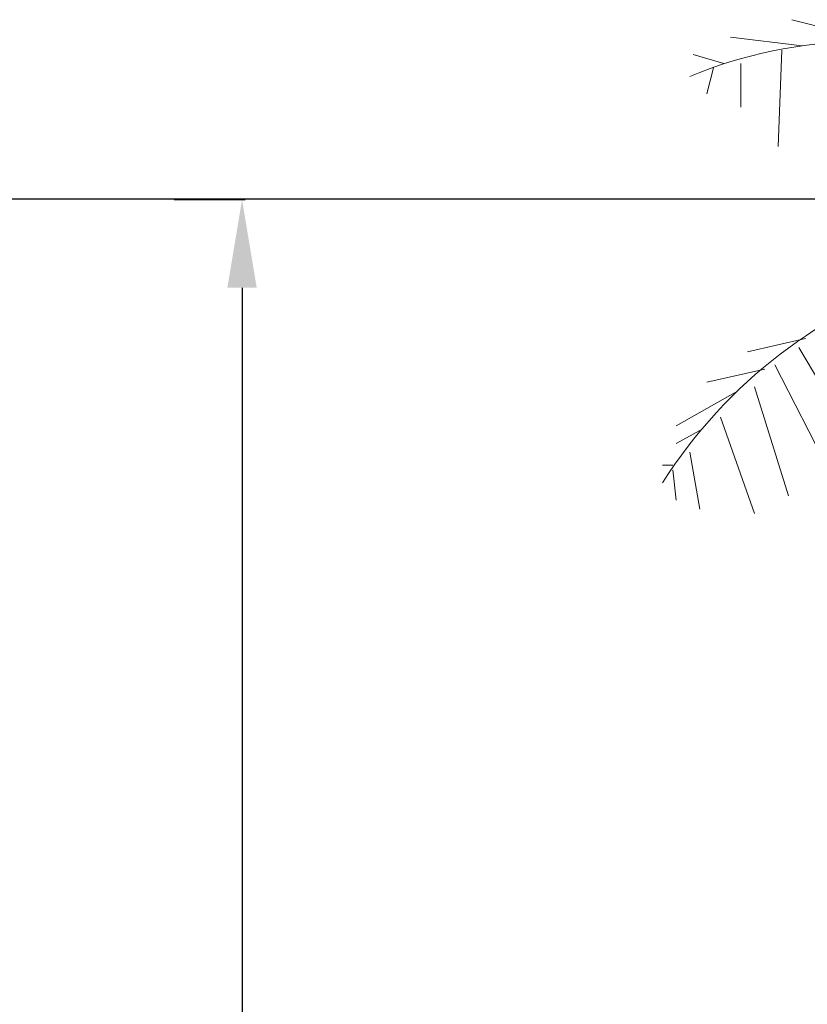
# Model space of a CAD drawing. Units: inches. Extents: x -301 to 715, y -607 to 364.
# Tile 51 of 141: x 150 to 194, y -370 to -314. Entities that reach past the tile are written whole.
import ezdxf

# ---------------------------------------------------------------- set-up
doc = ezdxf.new("R2010")
doc.units = ezdxf.units.IN
doc.header["$MEASUREMENT"] = 0
doc.layers.add('A-ANNO-DIMS', color=2, linetype='Continuous', lineweight=18)
doc.layers.add('L-PLNT', color=94, linetype='Continuous', lineweight=13)
doc.styles.get("Standard").update_dxf_attribs({"font": 'arial.ttf'})
doc.dimstyles.get("Standard").update_dxf_attribs({"dimtxt": 0.18, "dimasz": 0.18, "dimexe": 0.18, "dimexo": 0.0625, "dimgap": 0.09, "dimtad": 0, "dimtih": 1, "dimtoh": 1, "dimdec": 1, "dimzin": 0, "dimdsep": 46, "dimlunit": 4, "dimtxsty": 'Standard', "dimcen": 0.09, "dimclrd": 3, "dimclre": 4, "dimclrt": 6, "dimadec": 0, "dimazin": 0, "dimtfac": 1, "dimtdec": 1, "dimtofl": 0, "dimtmove": 0, "dimatfit": 3, "dimfxl": 1, "dimtfill": 2, "dimtfillclr": 51, "dimtolj": 1, "dimtzin": 0, "dimarcsym": 0})

# ---------------------------------------------------------------- blocks, each defined once
blk = doc.blocks.new('*U34')
for p, q in [((-20.064, 191.751), (-25.863, 193.238)), ((-25.283, 191.751), (-29.342, 192.246)), ((-29.729, 190.759), (-31.469, 191.255)), ((-26.443, 191.503), (-26.636, 186.051)), ((-30.309, 190.512), (-30.695, 189.025)), ((-28.763, 190.759), (-28.763, 188.281)), ((-25.09, 175.148), (-28.376, 174.404)), ((-25.476, 174.652), (-21.224, 167.466)), ((-27.409, 173.413), (-30.695, 172.67)), ((-26.829, 173.661), (-23.544, 167.218)), ((-28.956, 172.174), (-32.435, 170.192)), ((-27.989, 172.422), (-26.056, 166.227)), ((-29.922, 170.687), (-27.989, 165.235)), ((-31.082, 169.944), (-32.435, 169.2)), ((-31.662, 168.705), (-31.082, 165.483)), ((-32.628, 167.961), (-33.208, 167.961)), ((-32.628, 167.713), (-32.435, 165.979))]:
    blk.add_line(p, q)
for centre, radius, start, end in [((-21.738, 166.094), 25.899, 27.6712, 112.5305), ((-9.259, 151.732), 28.386, 68.3831, 147.5322)]:
    blk.add_arc(centre, radius, start, end)
blk = doc.blocks.new('*D76')
at = {"layer": 'A-ANNO-DIMS', "color": 0, "lineweight": -2, "transparency": 16777216}
for p, q in [((158.28, -324.519), (162.311, -324.519)), ((162.131, -329.519), (162.131, -400.354)), ((162.131, -476.477), (162.131, -405.643)), ((158.28, -481.477), (162.311, -481.477))]:
    blk.add_line(p, q, dxfattribs=at)
at = {"layer": 'A-ANNO-DIMS', "color": 0, "transparency": 16777216}
for points in [[(161.297, -329.519), (162.964, -329.519), (162.131, -324.519)], [(161.297, -476.477), (162.964, -476.477), (162.131, -481.477)]]:
    blk.add_solid(points, dxfattribs=at)
at = {"layer": 'Defpoints', "color": 0, "transparency": 16777216}
for p in [(158.218, -324.519), (162.131, -324.519), (158.218, -481.477)]:
    blk.add_point(p, dxfattribs=at)
at = {"layer": 'A-ANNO-DIMS', "color": 0, "transparency": 16777216, "insert": (162.131, -402.998), "char_height": 5, "attachment_point": 5, "bg_fill": 1, "box_fill_scale": 1.25, "bg_fill_color": 51, "bg_fill_transparency": 0}
blk.add_mtext('\\A1;13\'-1"', dxfattribs=at)
blk = doc.blocks.new('*D176')
at = {"layer": 'A-ANNO-DIMS', "color": 4, "lineweight": -2, "transparency": 16777216}
for p, q in [((148.28, -324.477), (215.605, -324.477)), ((-15.22, -540.477), (215.605, -540.477))]:
    blk.add_line(p, q, dxfattribs=at)
at = {"layer": 'A-ANNO-DIMS', "color": 3, "lineweight": -2, "transparency": 16777216}
for p, q in [((215.425, -324.657), (215.425, -432.296)), ((215.425, -540.297), (215.425, -432.659))]:
    blk.add_line(p, q, dxfattribs=at)
at = {"layer": 'A-ANNO-DIMS', "color": 3, "transparency": 16777216}
for points in [[(215.395, -324.657), (215.455, -324.657), (215.425, -324.477)], [(215.395, -540.297), (215.455, -540.297), (215.425, -540.477)]]:
    blk.add_solid(points, dxfattribs=at)
at = {"layer": 'Defpoints', "color": 0, "transparency": 16777216}
for p in [(148.218, -324.477), (-15.282, -540.477), (215.425, -540.477)]:
    blk.add_point(p, dxfattribs=at)
at = {"layer": 'A-ANNO-DIMS', "color": 6, "transparency": 16777216, "insert": (215.425, -432.477), "char_height": 0.18, "attachment_point": 5, "bg_fill": 1, "box_fill_scale": 1.25, "bg_fill_color": 51, "bg_fill_transparency": 0}
blk.add_mtext('\\A1;18\'-0"', dxfattribs=at)

msp = doc.modelspace()

# ---------------------------------------------------------------- block references
at = {"layer": 'L-PLNT'}
msp.add_blockref('*U34', (219.184, -507.552), dxfattribs=at)

# ---------------------------------------------------------------- dimensions: what is measured, and where the dimension line sits
at = {"layer": 'A-ANNO-DIMS'}
for base, p1, p2, override, picture, middle in [((215.425, -540.477), (148.218, -324.477), (-15.282, -540.477), {"dimdec": 1, "dimlfac": 1, "dimrnd": 0, "dimzin": 1, "dimdsep": 46, "dimlunit": 4, "dimfrac": 2}, '*D176', (215.425, -432.477)), ((162.131, -324.519), (158.218, -481.477), (158.218, -324.519), {"dimtxt": 5, "dimasz": 5, "dimclrd": 0, "dimclre": 0, "dimclrt": 0}, '*D76', (162.131, -402.998))]:
    dim = msp.add_linear_dim(base=base, p1=p1, p2=p2, angle=90, dimstyle='Standard', override=override, dxfattribs=at)
    dim.commit()
    dim.dimension.update_dxf_attribs({"geometry": picture, "text_midpoint": middle})

doc.saveas('drawing.dxf')
